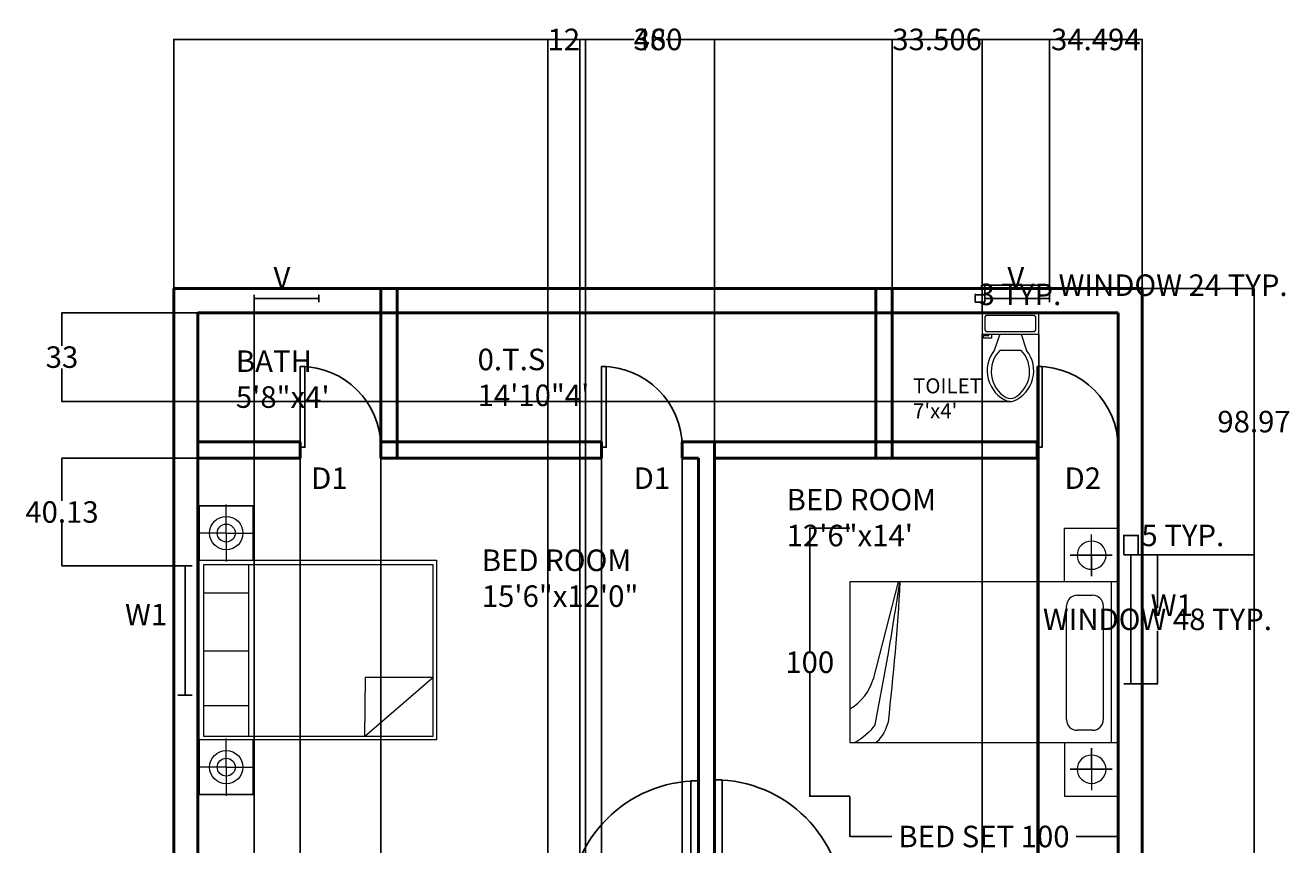
# Model space of a CAD drawing. Units: inches. Extents: x 3004 to 3478, y -798 to 114.
# Tile 5 of 5: x 3007 to 3477, y -190 to 114. Entities that reach past the tile are written whole.
import ezdxf

# ---------------------------------------------------------------- set-up
doc = ezdxf.new("R2010")
doc.units = ezdxf.units.IN
doc.header["$MEASUREMENT"] = 0
for name, color, linetype, lineweight in [('A-ANNO-DIMS', 2, 'Continuous', 18), ('A-ANNO-TEXT', 7, 'Continuous', 18), ('A-AREA-IDEN', 7, 'Continuous', 18), ('A-DOOR', 4, 'Continuous', 25), ('A-FLOR-FIXT', 9, 'Continuous', 18), ('A-FURN', 8, 'Continuous', 18), ('A-GLAZ', 4, 'Continuous', 25), ('A-WALL', 7, 'Continuous', 50)]:
    doc.layers.add(name, color=color, linetype=linetype, lineweight=lineweight)
doc.styles.get("Standard").update_dxf_attribs({"font": 'arial.ttf', "height": 8})
doc.dimstyles.get("Standard").update_dxf_attribs({"dimtxt": 0.18, "dimasz": 0.18, "dimexe": 0.18, "dimexo": 0.0625, "dimgap": 0.09, "dimtad": 0, "dimtih": 1, "dimtoh": 1, "dimzin": 0, "dimdsep": 46, "dimlunit": 4, "dimtxsty": 'Standard', "dimcen": 0.09, "dimadec": 0, "dimazin": 0, "dimtfac": 1, "dimtofl": 0, "dimtmove": 0, "dimatfit": 3, "dimfxl": 1, "dimtolj": 1, "dimtzin": 0, "dimarcsym": 0})

# ---------------------------------------------------------------- blocks, each defined once
blk = doc.blocks.new('*U14')
for p, q in [((9.5, -6), (9.5, -2)), ((-10, -8.5), (-8, -8.5)), ((-10, -9.5), (-10, -8.5)), ((-8, -8.5), (-8, -8)), ((-7, -8), (-7, -9.5)), ((-4, -8), (-6, -14)), ((4, -8), (6, -14)), ((-7, -9.5), (-10, -9.5)), ((4, -14), (-4, -14))]:
    blk.add_line(p, q)
blk.add_lwpolyline([(10.5, -8), (10.5, 0), (-10.5, 0), (-10.5, -8)], close=True)
for points in [[(-9.5, -2), (-9.5, -6)], [(8.5, -1), (-8.5, -1)], [(-8.5, -7), (8.5, -7)]]:
    blk.add_lwpolyline(points)
for centre, radius, start, end in [((-8.62, -1.88), 0.884, 81.8699, 188.1301), ((8.62, -1.88), 0.884, 351.8699, 98.1301), ((-8.62, -6.12), 0.884, 171.8699, 278.1301), ((8.62, -6.12), 0.884, 261.8699, 8.1301), ((3.52, -21.58), 12.17, 141.4691, 247.9714), ((4.2, -21.82), 11.33, 136.3677, 238.9468), ((-3.52, -21.58), 12.17, 292.0284, 38.5307), ((-4.2, -21.82), 11.33, 301.053, 43.6321), ((0, -27.88), 4, 245.7318, 294.2682), ((0, -29), 4, 254.8605, 285.1395)]:
    blk.add_arc(centre, radius, start, end)
blk = doc.blocks.new('A$C214F6537')
for p, q in [((0.465, 1.98, -0.169), (0.011, 1.98, -0.169)), ((0.011, 1.98, -0.169), (0.011, 1.53, -0.169)), ((0.011, 1.98, -0.169), (2.419, 1.98, -0.169)), ((0.011, 1.53, -0.169), (0.011, 1.98, -0.169)), ((0.238, 1.755, -0.439), (0.238, 1.993, -0.439)), ((0.465, 0, -0.169), (0.465, 1.98, -0.169)), ((0.465, 1.98, -0.169), (1.965, 1.98, -0.169)), ((0.465, 1.53, -0.169), (0.465, 1.98, -0.169)), ((0.495, 1.941, -0.169), (1.929, 1.941, -0.169)), ((0.495, 1.57, -0.169), (0.495, 1.941, -0.169)), ((0.752, 1.941, -0.169), (0.752, 1.57, -0.169)), ((1.209, 1.941, -0.169), (1.209, 1.57, -0.169)), ((1.694, 1.941, -0.169), (1.694, 1.57, -0.169)), ((1.929, 1.941, -0.169), (1.929, 1.57, -0.169)), ((1.965, 1.98, -0.169), (1.965, 0, -0.169)), ((2.419, 1.98, -0.169), (1.965, 1.98, -0.169)), ((1.965, 1.98, -0.169), (1.965, 1.53, -0.169)), ((2.192, 1.755, -0.439), (2.192, 1.993, -0.439)), ((2.419, 1.53, -0.169), (2.419, 1.98, -0.169)), ((2.419, 1.98, -0.169), (2.419, 1.53, -0.169)), ((0.238, 1.755, -0.439), (0, 1.755, -0.439)), ((0.238, 1.755, -0.439), (0.238, 1.517, -0.439)), ((0.238, 1.755, -0.439), (0.476, 1.755, -0.439)), ((2.192, 1.755, -0.439), (1.954, 1.755, -0.439)), ((2.192, 1.755, -0.439), (2.43, 1.755, -0.439)), ((2.192, 1.755, -0.439), (2.192, 1.517, -0.439)), ((0.011, 1.53, -0.169), (0.465, 1.53, -0.169)), ((0.465, 1.53, -0.169), (0.011, 1.53, -0.169)), ((0.465, 0, -0.169), (0.465, 1.53, -0.169)), ((0.495, 0.032, -0.169), (0.495, 1.57, -0.169)), ((1.929, 1.57, -0.169), (0.495, 1.57, -0.169)), ((1.929, 1.57, -0.169), (1.929, 0.032, -0.169)), ((1.965, 1.53, -0.169), (2.419, 1.53, -0.169)), ((2.419, 1.53, -0.169), (1.965, 1.53, -0.169)), ((1.965, 1.53, -0.169), (1.965, 0, -0.169)), ((0.495, 0.6, -0.169), (0.987, 0.032, -0.169)), ((0.987, 0.595, -0.169), (0.495, 0.6, -0.169)), ((0.987, 0.032, -0.169), (0.987, 0.595, -0.169)), ((1.965, 0, -0.169), (0.465, 0, -0.169)), ((1.965, 0, -0.169), (0.465, 0, -0.169)), ((1.929, 0.032, -0.169), (0.495, 0.032, -0.169))]:
    blk.add_line(p, q)
for centre, radius in [((0.238, 1.755, -0.439), 0.139), ((0.238, 1.755, -0.439), 0.075), ((2.192, 1.755, -0.439), 0.139), ((2.192, 1.755, -0.439), 0.075)]:
    blk.add_circle(centre, radius)
blk = doc.blocks.new('A$C1CF419FF')
for p, q in [((0, 1.6), (0, 2)), ((0, 2), (0.4, 2)), ((1.6, 2), (0.4, 2)), ((0.4, 2), (0.4, 0)), ((1.6, 0), (1.6, 2)), ((2, 2), (1.6, 2)), ((2, 1.6), (2, 2)), ((0.2016, 1.6438), (0.2016, 1.9558)), ((0.2016, 1.9558), (0.2016, 1.8029)), ((0.4024, 1.95), (1.6022, 1.95)), ((0.5802, 1.8901), (1.428, 1.8901)), ((1.7984, 1.6438), (1.7984, 1.9558)), ((1.7984, 1.9558), (1.7984, 1.8029)), ((0.3582, 1.8029), (0.0462, 1.8029)), ((0.2016, 1.8029), (0.3582, 1.8029)), ((0.2016, 1.8029), (0.2016, 1.6438)), ((0.5002, 1.6957), (0.5002, 1.8101)), ((1.508, 1.8101), (1.508, 1.6957)), ((1.7984, 1.8029), (1.6418, 1.8029)), ((1.6418, 1.8029), (1.9538, 1.8029)), ((1.7984, 1.8029), (1.7984, 1.6438)), ((1.428, 1.6157), (0.5802, 1.6157)), ((0.4, 1.6), (0, 1.6)), ((1.6, 1.6), (2, 1.6)), ((0.4, 0.3595), (1.1271, 0.1737)), ((0.4, 0), (1.6, 0))]:
    blk.add_line(p, q)
for centre, radius, start, end in [((0.5802, 1.8101), 0.08, 90, 180), ((1.428, 1.8101), 0.08, 0, 90), ((0.5802, 1.6957), 0.08, 180, 270), ((1.428, 1.6957), 0.08, 270, 0), ((1.0142, -0.1991), 0.3894, 30.74256, 73.15836)]:
    blk.add_arc(centre, radius, start, end)
blk.add_ellipse((0.2016, 1.8029), major_axis=(0, 0.1081), ratio=0.975448, start_param=3.141593, end_param=9.424778)
at = {"extrusion": (0, 0, -1)}
blk.add_ellipse((1.7984, 1.8029), major_axis=(0, -0.1081), ratio=0.975448, dxfattribs=at)
for centre, major_axis, ratio, start_param, end_param in [((-0.5372, -27.7974), (-0.2522, 28.1986), 0.804733, 0.052423, 0.098615), ((-1.0268, -20.3946), (-16.1576, 14.8127), 0.921097, 0.937065, 0.987694), ((1.3756, -0.1321), (0.0073, 0.4244), 0.825424, 0.18152, 0.67424), ((1.3503, -0.1021), (-0.1187, 0.3175), 0.834521, 0.831235, 1.457081)]:
    blk.add_ellipse(centre, major_axis=major_axis, ratio=ratio, start_param=start_param, end_param=end_param, dxfattribs=at)
blk = doc.blocks.new('*U16')
for p, q in [((0, 0), (0, -100)), ((750, 0), (750, -100))]:
    blk.add_line(p, q)
blk.add_lwpolyline([(0, 0), (0, 750), (43.75, 750), (43.75, 0)], close=True)
blk.add_arc((0, 0), 750, 0, 90)
blk = doc.blocks.new('*U17')
for p, q in [((-750, 0), (-750, -100)), ((0, 0), (0, -100))]:
    blk.add_line(p, q)
blk.add_lwpolyline([(0, 0), (0, 750), (-43.75, 750), (-43.75, 0)], close=True)
blk.add_arc((0, 0), 750, 90, 180)
blk = doc.blocks.new('Window - Imperial')
for p, q in [((0, 4), (0, 0)), ((36, 4), (36, 0)), ((0, 2), (36, 2))]:
    blk.add_line(p, q)
blk = doc.blocks.new('*D20')
at = {"layer": 'A-ANNO-DIMS', "color": 0, "lineweight": -2, "transparency": 16777216}
for p, q in [((3420.72, -82.64), (3428.04, -82.64)), ((3427.86, -82.82), (3427.86, -102.42)), ((3427.86, -130.46), (3427.86, -110.87)), ((3420.72, -130.64), (3428.04, -130.64))]:
    blk.add_line(p, q, dxfattribs=at)
at = {"layer": 'A-ANNO-DIMS', "color": 0, "transparency": 16777216}
for points in [[(3427.83, -82.82), (3427.89, -82.82), (3427.86, -82.64)], [(3427.83, -130.46), (3427.89, -130.46), (3427.86, -130.64)]]:
    blk.add_solid(points, dxfattribs=at)
at = {"layer": 'Defpoints', "color": 0, "transparency": 16777216}
for p in [(3420.66, -82.64), (3420.66, -130.64), (3427.86, -130.64)]:
    blk.add_point(p, dxfattribs=at)
at = {"layer": 'A-ANNO-DIMS', "color": 0, "transparency": 16777216, "insert": (3427.86, -106.64), "char_height": 8, "attachment_point": 5}
blk.add_mtext('\\A1;WINDOW 48 TYP.', dxfattribs=at)
blk = doc.blocks.new('*D21')
at = {"layer": 'A-ANNO-DIMS', "color": 0, "lineweight": -2, "transparency": 16777216}
for p, q in [((3415.33, -82.58), (3415.33, -75.26)), ((3415.51, -75.44), (3420.48, -75.44)), ((3420.66, -82.58), (3420.66, -75.26)), ((3420.66, -75.44), (3420.84, -75.44))]:
    blk.add_line(p, q, dxfattribs=at)
at = {"layer": 'A-ANNO-DIMS', "color": 0, "transparency": 16777216}
for points in [[(3415.51, -75.41), (3415.51, -75.47), (3415.33, -75.44)], [(3420.48, -75.41), (3420.48, -75.47), (3420.66, -75.44)]]:
    blk.add_solid(points, dxfattribs=at)
at = {"layer": 'Defpoints', "color": 0, "transparency": 16777216}
for p in [(3420.66, -75.44), (3415.33, -82.64), (3420.66, -82.64)]:
    blk.add_point(p, dxfattribs=at)
at = {"layer": 'A-ANNO-DIMS', "color": 0, "transparency": 16777216, "insert": (3437.29, -75.44), "char_height": 8, "attachment_point": 5}
blk.add_mtext('\\A1;5 TYP.', dxfattribs=at)
blk = doc.blocks.new('*D22')
at = {"layer": 'A-ANNO-DIMS', "color": 0, "lineweight": -2, "transparency": 16777216}
for p, q in [((3363.72, 14.01), (3363.72, 17.73)), ((3363.9, 17.55), (3387.54, 17.55)), ((3387.72, 14.01), (3387.72, 17.73)), ((3387.72, 17.55), (3387.9, 17.55))]:
    blk.add_line(p, q, dxfattribs=at)
at = {"layer": 'A-ANNO-DIMS', "color": 0, "transparency": 16777216}
for points in [[(3363.9, 17.58), (3363.9, 17.52), (3363.72, 17.55)], [(3387.54, 17.58), (3387.54, 17.52), (3387.72, 17.55)]]:
    blk.add_solid(points, dxfattribs=at)
at = {"layer": 'Defpoints', "color": 0, "transparency": 16777216}
for p in [(3387.72, 17.55), (3363.72, 13.95), (3387.72, 13.95)]:
    blk.add_point(p, dxfattribs=at)
at = {"layer": 'A-ANNO-DIMS', "color": 0, "transparency": 16777216, "insert": (3433.69, 17.55), "char_height": 8, "attachment_point": 5}
blk.add_mtext('\\A1;WINDOW 24 TYP.', dxfattribs=at)
blk = doc.blocks.new('*D23')
at = {"layer": 'A-ANNO-DIMS', "color": 0, "lineweight": -2, "transparency": 16777216}
for p, q in [((3360.12, 13.95), (3360.12, 14.13)), ((3360.12, 14.13), (3360.3, 14.13)), ((3363.66, 13.95), (3359.94, 13.95)), ((3363.66, 11.28), (3359.94, 11.28)), ((3360.12, 11.46), (3360.12, 13.77))]:
    blk.add_line(p, q, dxfattribs=at)
at = {"layer": 'A-ANNO-DIMS', "color": 0, "transparency": 16777216}
for points in [[(3360.09, 13.77), (3360.15, 13.77), (3360.12, 13.95)], [(3360.09, 11.46), (3360.15, 11.46), (3360.12, 11.28)]]:
    blk.add_solid(points, dxfattribs=at)
at = {"layer": 'Defpoints', "color": 0, "transparency": 16777216}
for p in [(3360.12, 13.95), (3363.72, 13.95), (3363.72, 11.28)]:
    blk.add_point(p, dxfattribs=at)
at = {"layer": 'A-ANNO-DIMS', "color": 0, "transparency": 16777216, "insert": (3376.75, 14.13), "char_height": 8, "attachment_point": 5}
blk.add_mtext('\\A1;3 TYP.', dxfattribs=at)
blk = doc.blocks.new('*D34')
at = {"layer": 'A-ANNO-DIMS', "color": 0, "lineweight": -2, "transparency": 16777216}
for p, q in [((3313.57, -172.46), (3313.57, -187.52)), ((3413.21, -172.46), (3413.21, -187.52)), ((3313.75, -187.34), (3329.19, -187.34)), ((3413.03, -187.34), (3397.59, -187.34))]:
    blk.add_line(p, q, dxfattribs=at)
at = {"layer": 'A-ANNO-DIMS', "color": 0, "transparency": 16777216}
for points in [[(3313.75, -187.31), (3313.75, -187.37), (3313.57, -187.34)], [(3413.03, -187.31), (3413.03, -187.37), (3413.21, -187.34)]]:
    blk.add_solid(points, dxfattribs=at)
at = {"layer": 'Defpoints', "color": 0, "transparency": 16777216}
for p in [(3313.57, -172.39), (3413.21, -172.39), (3413.21, -187.34)]:
    blk.add_point(p, dxfattribs=at)
at = {"layer": 'A-ANNO-DIMS', "color": 0, "transparency": 16777216, "insert": (3363.39, -187.34), "char_height": 8, "attachment_point": 5}
blk.add_mtext('\\A1;BED SET 100', dxfattribs=at)
blk = doc.blocks.new('*D35')
at = {"layer": 'A-ANNO-DIMS', "color": 0, "lineweight": -2, "transparency": 16777216}
for p, q in [((3313.51, -72.75), (3298.44, -72.75)), ((3298.62, -72.93), (3298.62, -118.4)), ((3298.62, -172.21), (3298.62, -126.75)), ((3313.51, -172.39), (3298.44, -172.39))]:
    blk.add_line(p, q, dxfattribs=at)
at = {"layer": 'A-ANNO-DIMS', "color": 0, "transparency": 16777216}
for points in [[(3298.59, -72.93), (3298.65, -72.93), (3298.62, -72.75)], [(3298.59, -172.21), (3298.65, -172.21), (3298.62, -172.39)]]:
    blk.add_solid(points, dxfattribs=at)
at = {"layer": 'Defpoints', "color": 0, "transparency": 16777216}
for p in [(3313.57, -72.75), (3298.62, -172.39), (3313.57, -172.39)]:
    blk.add_point(p, dxfattribs=at)
at = {"layer": 'A-ANNO-DIMS', "color": 0, "transparency": 16777216, "insert": (3298.62, -122.57), "char_height": 8, "attachment_point": 5}
blk.add_mtext('\\A1;100', dxfattribs=at)
blk = doc.blocks.new('*D38')
at = {"layer": 'A-ANNO-DIMS', "color": 0, "lineweight": -2, "transparency": 16777216}
for p, q in [((3062.21, 16.38), (3062.21, 109.05)), ((3062.39, 108.87), (3233.3, 108.87)), ((3422.03, 108.87), (3251.12, 108.87)), ((3422.21, 16.38), (3422.21, 109.05))]:
    blk.add_line(p, q, dxfattribs=at)
at = {"layer": 'A-ANNO-DIMS', "color": 0, "transparency": 16777216}
for points in [[(3062.39, 108.9), (3062.39, 108.84), (3062.21, 108.87)], [(3422.03, 108.9), (3422.03, 108.84), (3422.21, 108.87)]]:
    blk.add_solid(points, dxfattribs=at)
at = {"layer": 'Defpoints', "color": 0, "transparency": 16777216}
for p in [(3422.21, 108.87), (3062.21, 16.32), (3422.21, 16.32)]:
    blk.add_point(p, dxfattribs=at)
at = {"layer": 'A-ANNO-DIMS', "color": 0, "transparency": 16777216, "insert": (3242.21, 108.87), "char_height": 8, "attachment_point": 5}
blk.add_mtext('\\A1;360', dxfattribs=at)
blk = doc.blocks.new('*D39')
at = {"layer": 'A-ANNO-DIMS', "color": 0, "lineweight": -2, "transparency": 16777216}
for p, q in [((3422.27, 16.32), (3463.94, 16.32)), ((3463.76, 16.14), (3463.76, -363.5)), ((3463.76, -751.5), (3463.76, -371.85)), ((3422.27, -751.68), (3463.94, -751.68))]:
    blk.add_line(p, q, dxfattribs=at)
at = {"layer": 'A-ANNO-DIMS', "color": 0, "transparency": 16777216}
for points in [[(3463.73, 16.14), (3463.79, 16.14), (3463.76, 16.32)], [(3463.73, -751.5), (3463.79, -751.5), (3463.76, -751.68)]]:
    blk.add_solid(points, dxfattribs=at)
at = {"layer": 'Defpoints', "color": 0, "transparency": 16777216}
for p in [(3422.21, 16.32), (3422.21, -751.68), (3463.76, -751.68)]:
    blk.add_point(p, dxfattribs=at)
at = {"layer": 'A-ANNO-DIMS', "color": 0, "transparency": 16777216, "insert": (3463.76, -367.68), "char_height": 8, "attachment_point": 5}
blk.add_mtext('\\A1;768', dxfattribs=at)
blk = doc.blocks.new('*D45')
at = {"layer": 'A-ANNO-DIMS', "color": 0, "lineweight": -2, "transparency": 16777216}
for p, q in [((3422.21, 16.26), (3422.21, -793.41)), ((3413.21, 7.26), (3413.21, -793.41)), ((3413.39, -793.23), (3414.99, -793.23)), ((3422.03, -793.23), (3420.43, -793.23))]:
    blk.add_line(p, q, dxfattribs=at)
at = {"layer": 'A-ANNO-DIMS', "color": 0, "transparency": 16777216}
for points in [[(3413.39, -793.2), (3413.39, -793.26), (3413.21, -793.23)], [(3422.03, -793.2), (3422.03, -793.26), (3422.21, -793.23)]]:
    blk.add_solid(points, dxfattribs=at)
at = {"layer": 'Defpoints', "color": 0, "transparency": 16777216}
for p in [(3422.21, 16.32), (3413.21, 7.32), (3422.21, -793.23)]:
    blk.add_point(p, dxfattribs=at)
at = {"layer": 'A-ANNO-DIMS', "color": 0, "transparency": 16777216, "insert": (3417.71, -793.23), "char_height": 8, "attachment_point": 5}
blk.add_mtext('\\A1;9', dxfattribs=at)
blk = doc.blocks.new('*D47')
at = {"layer": 'A-ANNO-DIMS', "color": 0, "lineweight": -2, "transparency": 16777216}
for p, q in [((3383.21, -46.74), (3383.21, -793.41)), ((3413.21, -42.74), (3413.21, -793.41)), ((3383.39, -793.23), (3392.41, -793.23)), ((3413.03, -793.23), (3404.01, -793.23))]:
    blk.add_line(p, q, dxfattribs=at)
at = {"layer": 'A-ANNO-DIMS', "color": 0, "transparency": 16777216}
for points in [[(3383.39, -793.2), (3383.39, -793.26), (3383.21, -793.23)], [(3413.03, -793.2), (3413.03, -793.26), (3413.21, -793.23)]]:
    blk.add_solid(points, dxfattribs=at)
at = {"layer": 'Defpoints', "color": 0, "transparency": 16777216}
for p in [(3383.21, -46.68), (3413.21, -42.68), (3413.21, -793.23)]:
    blk.add_point(p, dxfattribs=at)
at = {"layer": 'A-ANNO-DIMS', "color": 0, "transparency": 16777216, "insert": (3398.21, -793.23), "char_height": 8, "attachment_point": 5}
blk.add_mtext('\\A1;30', dxfattribs=at)
blk = doc.blocks.new('*D48')
at = {"layer": 'A-ANNO-DIMS', "color": 0, "lineweight": -2, "transparency": 16777216}
for p, q in [((3422.27, 16.32), (3463.94, 16.32)), ((3463.76, 16.14), (3463.76, -28.99)), ((3463.76, -82.46), (3463.76, -37.34)), ((3415.39, -82.64), (3463.94, -82.64))]:
    blk.add_line(p, q, dxfattribs=at)
at = {"layer": 'A-ANNO-DIMS', "color": 0, "transparency": 16777216}
for points in [[(3463.73, 16.14), (3463.79, 16.14), (3463.76, 16.32)], [(3463.73, -82.46), (3463.79, -82.46), (3463.76, -82.64)]]:
    blk.add_solid(points, dxfattribs=at)
at = {"layer": 'Defpoints', "color": 0, "transparency": 16777216}
for p in [(3422.21, 16.32), (3415.33, -82.64), (3463.76, -82.64)]:
    blk.add_point(p, dxfattribs=at)
at = {"layer": 'A-ANNO-DIMS', "color": 0, "transparency": 16777216, "insert": (3463.76, -33.16), "char_height": 8, "attachment_point": 5}
blk.add_mtext('\\A1;98.97', dxfattribs=at)
blk = doc.blocks.new('*D49')
at = {"layer": 'A-ANNO-DIMS', "color": 0, "lineweight": -2, "transparency": 16777216}
for p, q in [((3071.15, -46.68), (3020.48, -46.68)), ((3020.66, -46.86), (3020.66, -62.57)), ((3020.66, -86.63), (3020.66, -70.92)), ((3063.72, -86.81), (3020.48, -86.81))]:
    blk.add_line(p, q, dxfattribs=at)
at = {"layer": 'A-ANNO-DIMS', "color": 0, "transparency": 16777216}
for points in [[(3020.63, -46.86), (3020.69, -46.86), (3020.66, -46.68)], [(3020.63, -86.63), (3020.69, -86.63), (3020.66, -86.81)]]:
    blk.add_solid(points, dxfattribs=at)
at = {"layer": 'Defpoints', "color": 0, "transparency": 16777216}
for p in [(3071.21, -46.68), (3020.66, -86.81), (3063.78, -86.81)]:
    blk.add_point(p, dxfattribs=at)
at = {"layer": 'A-ANNO-DIMS', "color": 0, "transparency": 16777216, "insert": (3020.66, -66.74), "char_height": 8, "attachment_point": 5}
blk.add_mtext('\\A1;40.13', dxfattribs=at)
blk = doc.blocks.new('*D53')
at = {"layer": 'A-ANNO-DIMS', "color": 0, "lineweight": -2, "transparency": 16777216}
for p, q in [((3092.13, 11.22), (3092.13, -793.41)), ((3071.21, 7.26), (3071.21, -793.41)), ((3071.39, -793.23), (3091.95, -793.23)), ((3092.13, -793.23), (3092.31, -793.23))]:
    blk.add_line(p, q, dxfattribs=at)
at = {"layer": 'A-ANNO-DIMS', "color": 0, "transparency": 16777216}
for points in [[(3071.39, -793.2), (3071.39, -793.26), (3071.21, -793.23)], [(3091.95, -793.2), (3091.95, -793.26), (3092.13, -793.23)]]:
    blk.add_solid(points, dxfattribs=at)
at = {"layer": 'Defpoints', "color": 0, "transparency": 16777216}
for p in [(3092.13, 11.28), (3071.21, 7.32), (3092.13, -793.23)]:
    blk.add_point(p, dxfattribs=at)
at = {"layer": 'A-ANNO-DIMS', "color": 0, "transparency": 16777216, "insert": (3105.93, -793.23), "char_height": 8, "attachment_point": 5}
blk.add_mtext('\\A1;20.92', dxfattribs=at)
blk = doc.blocks.new('*D54')
at = {"layer": 'A-ANNO-DIMS', "color": 0, "lineweight": -2, "transparency": 16777216}
for p, q in [((3387.72, 11.35), (3387.72, 109.05)), ((3387.9, 108.87), (3388.29, 108.87)), ((3422.03, 108.87), (3421.64, 108.87)), ((3422.21, 16.38), (3422.21, 109.05))]:
    blk.add_line(p, q, dxfattribs=at)
at = {"layer": 'A-ANNO-DIMS', "color": 0, "transparency": 16777216}
for points in [[(3387.9, 108.9), (3387.9, 108.84), (3387.72, 108.87)], [(3422.03, 108.9), (3422.03, 108.84), (3422.21, 108.87)]]:
    blk.add_solid(points, dxfattribs=at)
at = {"layer": 'Defpoints', "color": 0, "transparency": 16777216}
for p in [(3387.72, 108.87), (3422.21, 16.32), (3387.72, 11.28)]:
    blk.add_point(p, dxfattribs=at)
at = {"layer": 'A-ANNO-DIMS', "color": 0, "transparency": 16777216, "insert": (3404.96, 108.87), "char_height": 8, "attachment_point": 5}
blk.add_mtext('\\A1;34.494', dxfattribs=at)
blk = doc.blocks.new('*D55')
at = {"layer": 'A-ANNO-DIMS', "color": 0, "lineweight": -2, "transparency": 16777216}
for p, q in [((3215.21, -494.62), (3215.21, 109.05)), ((3215.39, 108.87), (3233.22, 108.87)), ((3263.03, 108.87), (3245.2, 108.87)), ((3263.21, -494.62), (3263.21, 109.05))]:
    blk.add_line(p, q, dxfattribs=at)
at = {"layer": 'A-ANNO-DIMS', "color": 0, "transparency": 16777216}
for points in [[(3215.39, 108.9), (3215.39, 108.84), (3215.21, 108.87)], [(3263.03, 108.9), (3263.03, 108.84), (3263.21, 108.87)]]:
    blk.add_solid(points, dxfattribs=at)
at = {"layer": 'Defpoints', "color": 0, "transparency": 16777216}
for p in [(3263.21, 108.87), (3215.21, -494.68), (3263.21, -494.68)]:
    blk.add_point(p, dxfattribs=at)
at = {"layer": 'A-ANNO-DIMS', "color": 0, "transparency": 16777216, "insert": (3239.21, 108.87), "char_height": 8, "attachment_point": 5}
blk.add_mtext('\\A1;48', dxfattribs=at)
blk = doc.blocks.new('*D57')
at = {"layer": 'A-ANNO-DIMS', "color": 0, "lineweight": -2, "transparency": 16777216}
for p, q in [((3201.21, -644.62), (3201.21, 109.05)), ((3201.39, 108.87), (3201.81, 108.87)), ((3213.03, 108.87), (3212.61, 108.87)), ((3213.21, -644.62), (3213.21, 109.05))]:
    blk.add_line(p, q, dxfattribs=at)
at = {"layer": 'A-ANNO-DIMS', "color": 0, "transparency": 16777216}
for points in [[(3201.39, 108.9), (3201.39, 108.84), (3201.21, 108.87)], [(3213.03, 108.9), (3213.03, 108.84), (3213.21, 108.87)]]:
    blk.add_solid(points, dxfattribs=at)
at = {"layer": 'Defpoints', "color": 0, "transparency": 16777216}
for p in [(3213.21, 108.87), (3201.21, -644.68), (3213.21, -644.68)]:
    blk.add_point(p, dxfattribs=at)
at = {"layer": 'A-ANNO-DIMS', "color": 0, "transparency": 16777216, "insert": (3207.21, 108.87), "char_height": 8, "attachment_point": 5}
blk.add_mtext('\\A1;12', dxfattribs=at)
blk = doc.blocks.new('*D59')
at = {"layer": 'A-ANNO-DIMS', "color": 0, "lineweight": -2, "transparency": 16777216}
for p, q in [((3362.72, -0.74), (3362.72, -793.41)), ((3383.72, -0.74), (3383.72, -793.41)), ((3362.9, -793.23), (3368.1, -793.23)), ((3383.54, -793.23), (3378.33, -793.23))]:
    blk.add_line(p, q, dxfattribs=at)
at = {"layer": 'A-ANNO-DIMS', "color": 0, "transparency": 16777216}
for points in [[(3362.9, -793.2), (3362.9, -793.26), (3362.72, -793.23)], [(3383.54, -793.2), (3383.54, -793.26), (3383.72, -793.23)]]:
    blk.add_solid(points, dxfattribs=at)
at = {"layer": 'Defpoints', "color": 0, "transparency": 16777216}
for p in [(3362.72, -0.68), (3383.72, -0.68), (3383.72, -793.23)]:
    blk.add_point(p, dxfattribs=at)
at = {"layer": 'A-ANNO-DIMS', "color": 0, "transparency": 16777216, "insert": (3373.22, -793.23), "char_height": 8, "attachment_point": 5}
blk.add_mtext('\\A1;21', dxfattribs=at)
blk = doc.blocks.new('*D60')
at = {"layer": 'A-ANNO-DIMS', "color": 0, "lineweight": -2, "transparency": 16777216}
for p, q in [((3362.66, 7.32), (3020.48, 7.32)), ((3020.66, 7.14), (3020.66, -5)), ((3020.66, -25.5), (3020.66, -13.36)), ((3373.16, -25.68), (3020.48, -25.68))]:
    blk.add_line(p, q, dxfattribs=at)
at = {"layer": 'A-ANNO-DIMS', "color": 0, "transparency": 16777216}
for points in [[(3020.63, 7.14), (3020.69, 7.14), (3020.66, 7.32)], [(3020.63, -25.5), (3020.69, -25.5), (3020.66, -25.68)]]:
    blk.add_solid(points, dxfattribs=at)
at = {"layer": 'Defpoints', "color": 0, "transparency": 16777216}
for p in [(3362.72, 7.32), (3020.66, -25.68), (3373.22, -25.68)]:
    blk.add_point(p, dxfattribs=at)
at = {"layer": 'A-ANNO-DIMS', "color": 0, "transparency": 16777216, "insert": (3020.66, -9.18), "char_height": 8, "attachment_point": 5}
blk.add_mtext('\\A1;33', dxfattribs=at)
blk = doc.blocks.new('*D61')
at = {"layer": 'A-ANNO-DIMS', "color": 0, "lineweight": -2, "transparency": 16777216}
for p, q in [((3329.031316, 108.87211), (3328.851316, 108.87211)), ((3329.211316, 16.38461), (3329.211316, 109.05211)), ((3362.717698, 7.38461), (3362.717698, 109.05211)), ((3362.897698, 108.87211), (3363.077698, 108.87211))]:
    blk.add_line(p, q, dxfattribs=at)
at = {"layer": 'A-ANNO-DIMS', "color": 0, "transparency": 16777216}
for points in [[(3329.031316, 108.90211), (3329.031316, 108.84211), (3329.211316, 108.87211)], [(3362.897698, 108.90211), (3362.897698, 108.84211), (3362.717698, 108.87211)]]:
    blk.add_solid(points, dxfattribs=at)
at = {"layer": 'Defpoints', "color": 0, "transparency": 16777216}
for p in [(3362.717698, 108.87211), (3329.211316, 16.32211), (3362.717698, 7.32211)]:
    blk.add_point(p, dxfattribs=at)
at = {"layer": 'A-ANNO-DIMS', "color": 0, "transparency": 16777216, "insert": (3345.964507, 108.87211), "char_height": 8, "attachment_point": 5}
blk.add_mtext('\\A1;33.506', dxfattribs=at)
blk = doc.blocks.new('*D63')
at = {"layer": 'A-ANNO-DIMS', "color": 0, "lineweight": -2, "transparency": 16777216}
for p, q in [((3221.21, -46.74), (3221.21, -793.41)), ((3251.21, -46.74), (3251.21, -793.41)), ((3221.39, -793.23), (3230.41, -793.23)), ((3251.03, -793.23), (3242.01, -793.23))]:
    blk.add_line(p, q, dxfattribs=at)
at = {"layer": 'A-ANNO-DIMS', "color": 0, "transparency": 16777216}
for points in [[(3221.39, -793.2), (3221.39, -793.26), (3221.21, -793.23)], [(3251.03, -793.2), (3251.03, -793.26), (3251.21, -793.23)]]:
    blk.add_solid(points, dxfattribs=at)
at = {"layer": 'Defpoints', "color": 0, "transparency": 16777216}
for p in [(3221.21, -46.68), (3251.21, -46.68), (3251.21, -793.23)]:
    blk.add_point(p, dxfattribs=at)
at = {"layer": 'A-ANNO-DIMS', "color": 0, "transparency": 16777216, "insert": (3236.21, -793.23), "char_height": 8, "attachment_point": 5}
blk.add_mtext('\\A1;30', dxfattribs=at)
blk = doc.blocks.new('*D65')
at = {"layer": 'A-ANNO-DIMS', "color": 0, "lineweight": -2, "transparency": 16777216}
for p, q in [((3109.21, -46.74), (3109.21, -793.41)), ((3139.21, -46.74), (3139.21, -793.41)), ((3109.39, -793.23), (3118.41, -793.23)), ((3139.03, -793.23), (3130.01, -793.23))]:
    blk.add_line(p, q, dxfattribs=at)
at = {"layer": 'A-ANNO-DIMS', "color": 0, "transparency": 16777216}
for points in [[(3109.39, -793.2), (3109.39, -793.26), (3109.21, -793.23)], [(3139.03, -793.2), (3139.03, -793.26), (3139.21, -793.23)]]:
    blk.add_solid(points, dxfattribs=at)
at = {"layer": 'Defpoints', "color": 0, "transparency": 16777216}
for p in [(3109.21, -46.68), (3139.21, -46.68), (3139.21, -793.23)]:
    blk.add_point(p, dxfattribs=at)
at = {"layer": 'A-ANNO-DIMS', "color": 0, "transparency": 16777216, "insert": (3124.21, -793.23), "char_height": 8, "attachment_point": 5}
blk.add_mtext('\\A1;30', dxfattribs=at)

msp = doc.modelspace()

# ---------------------------------------------------------------- linework, layer by layer
at = {"layer": 'A-WALL'}
for p, q in [((3422.2113, 16.3221), (3062.2113, 16.3221)), ((3062.2113, 16.3221), (3062.2113, -703.6779)), ((3139.2113, 16.3221), (3139.2113, -46.6779)), ((3145.2113, 16.3221), (3145.2113, -46.6779)), ((3323.2113, 16.3221), (3323.2113, -46.6779)), ((3329.2113, 16.3221), (3329.2113, -46.6779)), ((3422.2113, 16.3221), (3422.2113, -703.6779)), ((3413.2113, 7.3221), (3071.2113, 7.3221)), ((3071.2113, 7.3221), (3071.2113, -703.6779)), ((3413.2113, 7.3221), (3413.2113, -703.6779)), ((3109.2113, -40.6779), (3071.2113, -40.6779)), ((3109.2113, -40.6779), (3109.2113, -46.6779)), ((3221.2113, -40.6779), (3139.2113, -40.6779)), ((3221.2113, -40.6779), (3221.2113, -46.6779)), ((3251.2113, -40.6779), (3251.2113, -46.6779)), ((3383.2113, -40.6779), (3251.2113, -40.6779)), ((3263.2113, -40.6779), (3263.2113, -220.6779)), ((3383.2113, -40.6779), (3383.2113, -46.6779)), ((3109.2113, -46.6779), (3071.2113, -46.6779)), ((3221.2113, -46.6779), (3139.2113, -46.6779)), ((3257.2113, -46.6779), (3251.2113, -46.6779)), ((3257.2113, -46.6779), (3257.2113, -220.6779)), ((3383.2113, -46.6779), (3263.2113, -46.6779))]:
    msp.add_line(p, q, dxfattribs=at)

# ---------------------------------------------------------------- block references
at = {"layer": 'A-DOOR'}
for name, p, xscale, yscale, zscale in [('*U16', (3109.2113, -42.6779), 0.0399999999999999, 0.0399999999999999, 0.0399999999999999), ('*U16', (3221.2113, -42.6779), 0.0399999999999999, 0.0399999999999999, 0.0399999999999999), ('*U16', (3383.2113, -42.6779), 0.0399999999999999, 0.0399999999999999, 0.0399999999999999), ('*U17', (3257.2113, -214.6779), 0.0639999999999998, 0.0639999999999998, 0.0639999999999998), ('*U16', (3263.2113, -214.2779), 0.0639999999999998, 0.0639999999999998, 0.0639999999999998)]:
    msp.add_blockref(name, p, dxfattribs=dict(at, xscale=xscale, yscale=yscale, zscale=zscale))
at = {"layer": 'A-FLOR-FIXT'}
msp.add_blockref('*U14', (3373.2177, 7.3221), dxfattribs=at)
at = {"layer": 'A-FURN'}
for name, p, xscale, yscale, zscale, rotation in [('A$C214F6537', (3159.8788, -172.174, 7.5147), 44.53130442995502, 44.53130442995502, 44.53130442995502, 90), ('A$C1CF419FF', (3313.5676, -72.7496), 49.82185608119661, 49.82185608119661, 49.82185608119661, 270)]:
    msp.add_blockref(name, p, dxfattribs=dict(at, xscale=xscale, yscale=yscale, zscale=zscale, rotation=rotation))
at = {"layer": 'A-GLAZ', "xscale": 0.6666666666666666, "yscale": 0.6666666666666666, "zscale": 0.6666666666666666}
for p in [(3092.1316, 11.284), (3363.7177, 11.284)]:
    msp.add_blockref('Window - Imperial', p, dxfattribs=at)
at = {"layer": 'A-GLAZ', "xscale": 1.333333333333333, "yscale": 1.333333333333333, "zscale": 1.333333333333333, "rotation": 270}
for p in [(3415.3269, -82.6443), (3063.7808, -86.8091)]:
    msp.add_blockref('Window - Imperial', p, dxfattribs=at)

# ---------------------------------------------------------------- texts
at = {"layer": 'A-ANNO-TEXT', "char_height": 8, "attachment_point": 1}
for s, width, insert in [('V', 54.295236, (3099.279, 24.3221)), ('V', 54.295236, (3372.0734, 24.3221)), ('D1', 22.083935, (3113.2806, -50.1786)), ('D1', 22.083935, (3233.1625, -50.1786)), ('D2', 22.083935, (3393.3235, -50.1786)), ('W1', 86.182133, (3425.3551, -97.3913)), ('W1', 86.182133, (3044.0997, -100.8725))]:
    msp.add_mtext_dynamic_manual_height_columns(s, width=width, gutter_width=40, heights=[0], dxfattribs=dict(at, insert=insert))
at = {"layer": 'A-AREA-IDEN', "attachment_point": 1}
for s, width, gutter_width, insert, char_height in [('BATH\\P5\'8"x4\'', 228.23715, 40, (3085.2934, -6.7022), 8), ('0.T.S\\P14\'10"4\'', 228.23715, 40, (3175.1538, -6.059), 8), ("TOILET\\P7'x4'", 159.072054, 27.8784, (3337.0113, -17.0695), 5.57568), ('BED ROOM\\P12\'6"x14\'', 228.23715, 40, (3290.0162, -58.1616), 8), ('BED ROOM\\P15\'6"x12\'0"', 228.23715, 40, (3176.7129, -80.675), 8)]:
    msp.add_mtext_dynamic_manual_height_columns(s, width=width, gutter_width=gutter_width, heights=[0], dxfattribs=dict(at, insert=insert, char_height=char_height))

# ---------------------------------------------------------------- dimensions: what is measured, and where the dimension line sits
at = {"layer": 'A-ANNO-DIMS'}
for base, p1, p2, override, picture, middle in [((3422.2113, 108.8721), (3062.2113, 16.3221), (3422.2113, 16.3221), {"dimdec": 0, "dimlfac": 1, "dimrnd": 0, "dimzin": 0, "dimdsep": 46, "dimlunit": 2}, '*D38', (3242.2113, 108.8721)), ((3213.2113, 108.8721), (3201.2113, -644.6779), (3213.2113, -644.6779), {"dimdec": 0, "dimlfac": 1, "dimrnd": 0, "dimzin": 0, "dimdsep": 46, "dimlunit": 2}, '*D57', (3207.2113, 108.8721)), ((3263.2113, 108.8721), (3215.2113, -494.6779), (3263.2113, -494.6779), {"dimdec": 0, "dimlfac": 1, "dimrnd": 0, "dimzin": 0, "dimdsep": 46, "dimlunit": 2}, '*D55', (3239.2113, 108.8721)), ((3362.7177, 108.8721), (3329.2113, 16.3221), (3362.7177, 7.3221), {"dimdec": 3, "dimlfac": 1, "dimrnd": 0, "dimzin": 0, "dimdsep": 46, "dimlunit": 2}, '*D61', (3345.9645, 108.8721)), ((3387.7177, 108.8721), (3422.2113, 16.3221), (3387.7177, 11.284), {"dimdec": 3, "dimlfac": 1, "dimrnd": 0, "dimzin": 0, "dimdsep": 46, "dimlunit": 2}, '*D54', (3404.9645, 108.8721)), ((3422.2113, -793.2279), (3413.2113, 7.3221), (3422.2113, 16.3221), {"dimdec": 0, "dimlfac": 1, "dimrnd": 0, "dimzin": 0, "dimdsep": 46, "dimlunit": 2}, '*D45', (3417.7113, -793.2279)), ((3092.1316, -793.2279), (3071.2113, 7.3221), (3092.1316, 11.284), {"dimdec": 2, "dimlfac": 1, "dimrnd": 0, "dimzin": 0, "dimdsep": 46, "dimlunit": 2}, '*D53', (3105.9268, -793.2279)), ((3383.7177, -793.2279), (3362.7177, -0.6779), (3383.7177, -0.6779), {"dimdec": 0, "dimlfac": 1, "dimrnd": 0, "dimzin": 0, "dimdsep": 46, "dimlunit": 2}, '*D59', (3373.2177, -793.2279)), ((3139.2113, -793.2279), (3109.2113, -46.6779), (3139.2113, -46.6779), {"dimdec": 0, "dimlfac": 1, "dimrnd": 0, "dimzin": 0, "dimdsep": 46, "dimlunit": 2}, '*D65', (3124.2113, -793.2279)), ((3251.2113, -793.2279), (3221.2113, -46.6779), (3251.2113, -46.6779), {"dimdec": 0, "dimlfac": 1, "dimrnd": 0, "dimzin": 0, "dimdsep": 46, "dimlunit": 2}, '*D63', (3236.2113, -793.2279)), ((3413.2113, -793.2279), (3383.2113, -46.6779), (3413.2113, -42.6779), {"dimdec": 0, "dimlfac": 1, "dimrnd": 0, "dimzin": 0, "dimdsep": 46, "dimlunit": 2}, '*D47', (3398.2113, -793.2279))]:
    dim = msp.add_linear_dim(base=base, p1=p1, p2=p2, dimstyle='Standard', override=override, dxfattribs=at)
    dim.commit()
    dim.dimension.update_dxf_attribs({"geometry": picture, "text_midpoint": middle})
for base, p1, p2, text, picture, middle in [((3387.7177, 17.5507), (3363.7177, 13.9507), (3387.7177, 13.9507), 'WINDOW <> TYP.', '*D22', (3433.693, 17.5507)), ((3420.6602, -75.4443), (3415.3269, -82.6443), (3420.6602, -82.6443), '<> TYP.', '*D21', (3437.2931, -75.4443)), ((3413.2113, -187.3399), (3313.5676, -172.3933), (3413.2113, -172.3933), 'BED SET <>', '*D34', (3363.3895, -187.3399))]:
    dim = msp.add_linear_dim(base=base, p1=p1, p2=p2, text=text, dimstyle='Standard', override={"dimdec": 0, "dimlfac": 1, "dimrnd": 0, "dimzin": 0, "dimdsep": 46, "dimlunit": 2}, dxfattribs=at)
    dim.commit()
    dim.dimension.update_dxf_attribs({"geometry": picture, "text_midpoint": middle})
for base, p1, p2, angle, text, picture, middle in [((3360.1177, 13.9507), (3363.7177, 11.284), (3363.7177, 13.9507), 90, '<> TYP.', '*D23', (3376.7479, 14.1307)), ((3427.8602, -130.6443), (3420.6602, -82.6443), (3420.6602, -130.6443), 270, 'WINDOW <> TYP.', '*D20', (3427.8602, -106.6443))]:
    dim = msp.add_linear_dim(base=base, p1=p1, p2=p2, angle=angle, text=text, dimstyle='Standard', override={"dimdec": 0, "dimlfac": 1, "dimrnd": 0, "dimzin": 0, "dimdsep": 46, "dimlunit": 2}, dxfattribs=at)
    dim.commit()
    dim.dimension.update_dxf_attribs({"geometry": picture, "text_midpoint": middle})
for base, p1, p2, angle, override, picture, middle in [((3463.7613, -82.6443), (3422.2113, 16.3221), (3415.3269, -82.6443), 90, {"dimdec": 2, "dimlfac": 1, "dimrnd": 0, "dimzin": 0, "dimdsep": 46, "dimlunit": 2}, '*D48', (3463.7613, -33.1611)), ((3463.7613, -751.6779), (3422.2113, 16.3221), (3422.2113, -751.6779), 90, {"dimdec": 0, "dimlfac": 1, "dimrnd": 0, "dimzin": 0, "dimdsep": 46, "dimlunit": 2}, '*D39', (3463.7613, -367.6779)), ((3020.6613, -25.6779), (3362.7177, 7.3221), (3373.2177, -25.6779), 90, {"dimdec": 0, "dimlfac": 1, "dimrnd": 0, "dimzin": 0, "dimdsep": 46, "dimlunit": 2}, '*D60', (3020.6613, -9.1779)), ((3020.6613, -86.8091), (3071.2113, -46.6779), (3063.7808, -86.8091), 90, {"dimdec": 2, "dimlfac": 1, "dimrnd": 0, "dimzin": 0, "dimdsep": 46, "dimlunit": 2}, '*D49', (3020.6613, -66.7435)), ((3298.621, -172.3933), (3313.5676, -72.7496), (3313.5676, -172.3933), 270, {"dimdec": 0, "dimlfac": 1, "dimrnd": 0, "dimzin": 0, "dimdsep": 46, "dimlunit": 2}, '*D35', (3298.621, -122.5714))]:
    dim = msp.add_linear_dim(base=base, p1=p1, p2=p2, angle=angle, dimstyle='Standard', override=override, dxfattribs=at)
    dim.commit()
    dim.dimension.update_dxf_attribs({"geometry": picture, "text_midpoint": middle})

doc.saveas('drawing.dxf')
